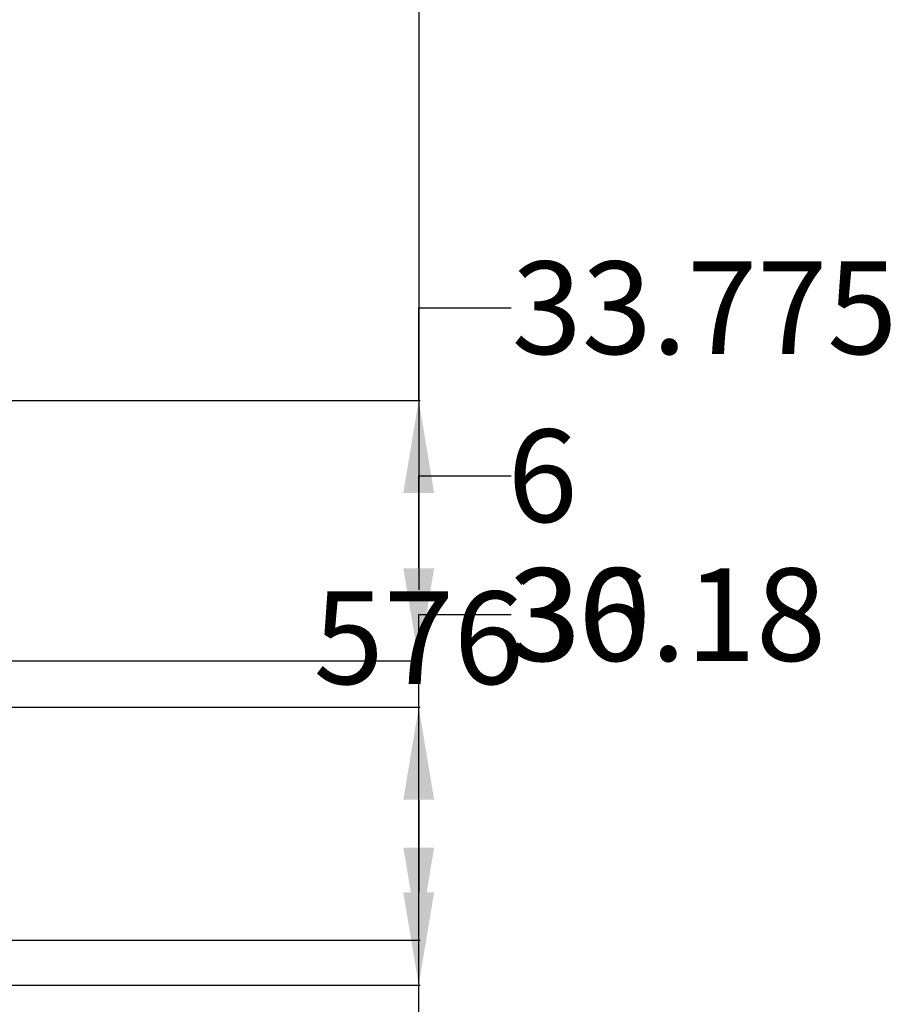
# Model space of a CAD drawing. Units: inches. Extents: x -77 to 516, y -119 to 536.
# Tile 10 of 11: x 403 to 516, y 159 to 287. Entities that reach past the tile are written whole.
import ezdxf

# ---------------------------------------------------------------- set-up
doc = ezdxf.new("R2010")
doc.units = ezdxf.units.IN
doc.header["$MEASUREMENT"] = 0
doc.layers.add('A-ANNO-DIMS', color=2, linetype='Continuous', lineweight=18)
doc.styles.get("Standard").update_dxf_attribs({"font": 'arial.ttf'})
doc.dimstyles.get("Standard").update_dxf_attribs({"dimtxt": 12, "dimasz": 12, "dimexe": 0.18, "dimexo": 0.0625, "dimgap": 0.09, "dimtad": 0, "dimtih": 1, "dimtoh": 1, "dimdec": 1, "dimzin": 0, "dimdsep": 46, "dimlunit": 4, "dimtxsty": 'Standard', "dimcen": 0.09, "dimadec": 0, "dimazin": 0, "dimtfac": 1, "dimtdec": 1, "dimtofl": 0, "dimtmove": 0, "dimatfit": 3, "dimfxl": 1, "dimtolj": 1, "dimtzin": 0, "dimarcsym": 0})

# ---------------------------------------------------------------- blocks, each defined once
blk = doc.blocks.new('*D37')
at = {"layer": 'A-ANNO-DIMS', "color": 0, "lineweight": -2, "transparency": 16777216}
for p, q in [((373.81, 494.59), (454.58, 494.59)), ((454.4, 482.59), (454.4, 212.81)), ((454.4, -69.41), (454.4, 200.37)), ((309, -81.41), (454.58, -81.41))]:
    blk.add_line(p, q, dxfattribs=at)
at = {"layer": 'A-ANNO-DIMS', "color": 0, "transparency": 16777216}
for points in [[(452.4, 482.59), (456.4, 482.59), (454.4, 494.59)], [(452.4, -69.41), (456.4, -69.41), (454.4, -81.41)]]:
    blk.add_solid(points, dxfattribs=at)
at = {"layer": 'Defpoints', "color": 0, "transparency": 16777216}
for p in [(373.75, 494.59), (454.4, 494.59), (308.93, -81.41)]:
    blk.add_point(p, dxfattribs=at)
at = {"layer": 'A-ANNO-DIMS', "color": 0, "transparency": 16777216, "insert": (454.4, 206.59), "char_height": 12, "attachment_point": 5}
blk.add_mtext('\\A1;576', dxfattribs=at)
blk = doc.blocks.new('*D42')
at = {"layer": 'A-ANNO-DIMS', "color": 0, "lineweight": -2, "transparency": 16777216}
for p, q in [((454.4, 197.59), (454.4, 209.59)), ((454.4, 209.59), (466.4, 209.59)), ((22.81, 197.59), (454.58, 197.59)), ((454.4, 179.41), (454.4, 185.59)), ((22.81, 167.41), (454.58, 167.41))]:
    blk.add_line(p, q, dxfattribs=at)
at = {"layer": 'A-ANNO-DIMS', "color": 0, "transparency": 16777216}
for points in [[(452.4, 185.59), (456.4, 185.59), (454.4, 197.59)], [(452.4, 179.41), (456.4, 179.41), (454.4, 167.41)]]:
    blk.add_solid(points, dxfattribs=at)
at = {"layer": 'Defpoints', "color": 0, "transparency": 16777216}
for p in [(22.75, 197.59), (454.4, 197.59), (22.75, 167.41)]:
    blk.add_point(p, dxfattribs=at)
at = {"layer": 'A-ANNO-DIMS', "color": 0, "transparency": 16777216, "insert": (486.75, 209.59), "char_height": 12, "attachment_point": 5}
blk.add_mtext('\\A1;30.18', dxfattribs=at)
blk = doc.blocks.new('*D43')
at = {"layer": 'A-ANNO-DIMS', "color": 0, "lineweight": -2, "transparency": 16777216}
for p, q in [((454.4, 237.36), (454.4, 249.36)), ((454.4, 249.36), (466.4, 249.36)), ((22.81, 237.36), (454.58, 237.36)), ((454.4, 215.59), (454.4, 225.36)), ((22.81, 203.59), (454.58, 203.59))]:
    blk.add_line(p, q, dxfattribs=at)
at = {"layer": 'A-ANNO-DIMS', "color": 0, "transparency": 16777216}
for points in [[(452.4, 225.36), (456.4, 225.36), (454.4, 237.36)], [(452.4, 215.59), (456.4, 215.59), (454.4, 203.59)]]:
    blk.add_solid(points, dxfattribs=at)
at = {"layer": 'Defpoints', "color": 0, "transparency": 16777216}
for p in [(22.75, 237.36), (454.4, 237.36), (22.75, 203.59)]:
    blk.add_point(p, dxfattribs=at)
at = {"layer": 'A-ANNO-DIMS', "color": 0, "transparency": 16777216, "insert": (491.44, 249.36), "char_height": 12, "attachment_point": 5}
blk.add_mtext('\\A1;33.775', dxfattribs=at)
blk = doc.blocks.new('*D55')
at = {"layer": 'A-ANNO-DIMS', "color": 0, "lineweight": -2, "transparency": 16777216}
for p, q in [((454.4, 197.59), (454.4, 209.59)), ((454.4, 209.59), (466.4, 209.59)), ((163.81, 197.59), (454.58, 197.59)), ((454.4, 173.59), (454.4, 185.59)), ((163.81, 161.59), (454.58, 161.59))]:
    blk.add_line(p, q, dxfattribs=at)
at = {"layer": 'A-ANNO-DIMS', "color": 0, "transparency": 16777216}
for points in [[(452.4, 185.59), (456.4, 185.59), (454.4, 197.59)], [(452.4, 173.59), (456.4, 173.59), (454.4, 161.59)]]:
    blk.add_solid(points, dxfattribs=at)
at = {"layer": 'Defpoints', "color": 0, "transparency": 16777216}
for p in [(163.75, 197.59), (454.4, 197.59), (163.75, 161.59)]:
    blk.add_point(p, dxfattribs=at)
at = {"layer": 'A-ANNO-DIMS', "color": 0, "transparency": 16777216, "insert": (475.08, 209.59), "char_height": 12, "attachment_point": 5}
blk.add_mtext('\\A1;36', dxfattribs=at)
blk = doc.blocks.new('*D56')
at = {"layer": 'A-ANNO-DIMS', "color": 0, "lineweight": -2, "transparency": 16777216}
for p, q in [((454.4, 215.59), (454.4, 227.59)), ((454.4, 227.59), (466.4, 227.59)), ((157.81, 203.59), (454.58, 203.59)), ((157.81, 197.59), (454.58, 197.59)), ((454.4, 185.59), (454.4, 173.59))]:
    blk.add_line(p, q, dxfattribs=at)
at = {"layer": 'A-ANNO-DIMS', "color": 0, "transparency": 16777216}
for points in [[(452.4, 215.59), (456.4, 215.59), (454.4, 203.59)], [(452.4, 185.59), (456.4, 185.59), (454.4, 197.59)]]:
    blk.add_solid(points, dxfattribs=at)
at = {"layer": 'Defpoints', "color": 0, "transparency": 16777216}
for p in [(157.75, 203.59), (454.4, 203.59), (157.75, 197.59)]:
    blk.add_point(p, dxfattribs=at)
at = {"layer": 'A-ANNO-DIMS', "color": 0, "transparency": 16777216, "insert": (470.45, 227.59), "char_height": 12, "attachment_point": 5}
blk.add_mtext('\\A1;6', dxfattribs=at)

msp = doc.modelspace()

# ---------------------------------------------------------------- dimensions: what is measured, and where the dimension line sits
at = {"layer": 'A-ANNO-DIMS'}
for base, p1, p2, override, picture, middle in [((454.4001, 494.5884), (308.9336, -81.4116), (373.7501, 494.5884), {"dimdec": 0, "dimlfac": 1, "dimrnd": 0, "dimzin": 0, "dimdsep": 46, "dimlunit": 2}, '*D37', (454.4001, 206.5884)), ((454.4001, 237.3631), (22.7501, 203.5884), (22.7501, 237.3631), {"dimdec": 3, "dimlfac": 1, "dimrnd": 0, "dimzin": 0, "dimdsep": 46, "dimlunit": 2}, '*D43', (491.4396, 249.3631)), ((454.4001, 203.5884), (157.7501, 197.5884), (157.7501, 203.5884), {"dimdec": 0, "dimlfac": 1, "dimrnd": 0, "dimzin": 0, "dimdsep": 46, "dimlunit": 2}, '*D56', (470.4519, 227.5884)), ((454.4001, 197.5884), (22.7501, 167.4079), (22.7501, 197.5884), {"dimdec": 2, "dimlfac": 1, "dimrnd": 0, "dimzin": 0, "dimdsep": 46, "dimlunit": 2}, '*D42', (486.7452, 209.5884)), ((454.4001, 197.5884), (163.7501, 161.5884), (163.7501, 197.5884), {"dimdec": 0, "dimlfac": 1, "dimrnd": 0, "dimzin": 0, "dimdsep": 46, "dimlunit": 2}, '*D55', (475.0767, 209.5884))]:
    dim = msp.add_linear_dim(base=base, p1=p1, p2=p2, angle=90, dimstyle='Standard', override=override, dxfattribs=at)
    dim.commit()
    dim.dimension.update_dxf_attribs({"geometry": picture, "text_midpoint": middle})

doc.saveas('drawing.dxf')
